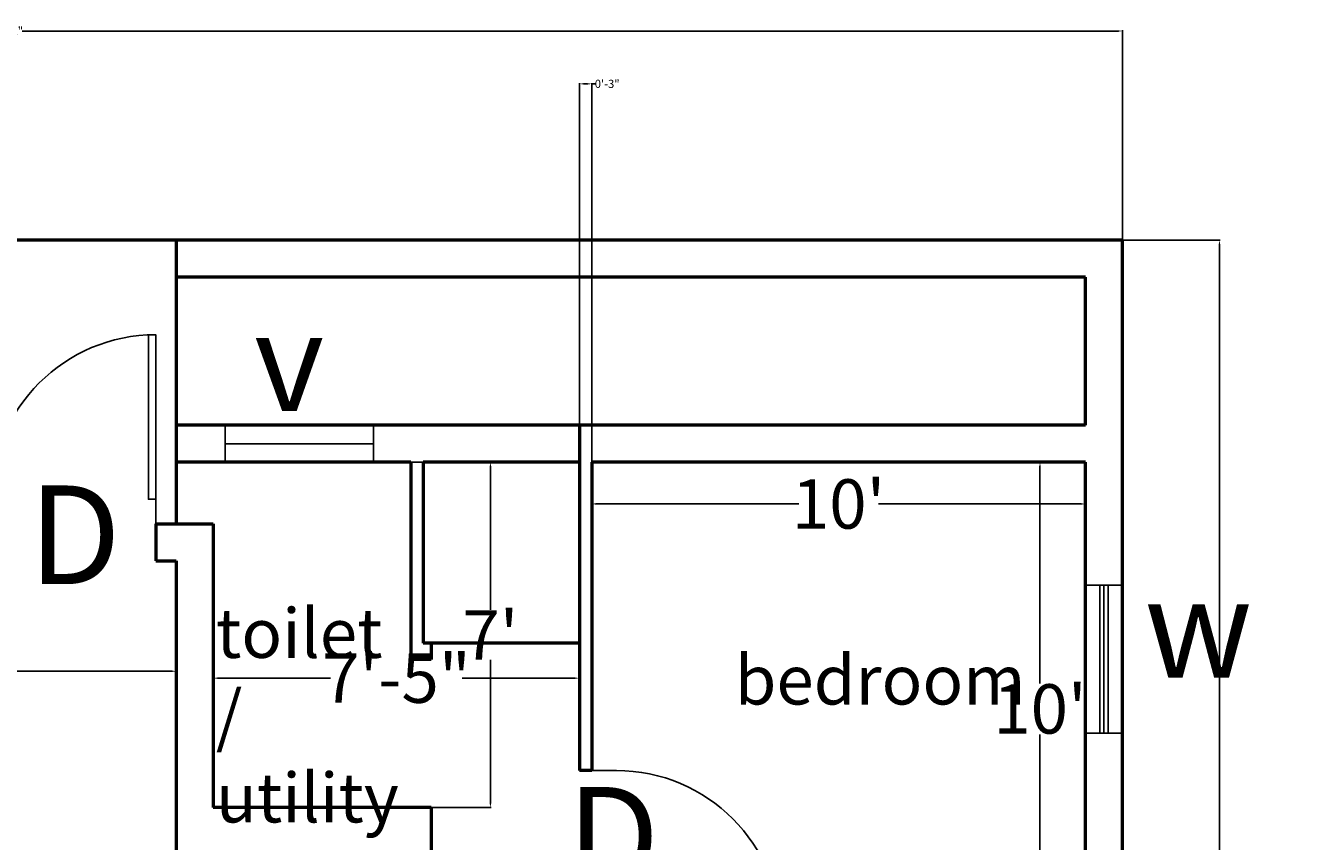
# Model space of a CAD drawing. Units: inches. Extents: x 409 to 7572, y 7 to 725.
# Tile 33 of 38: x 5952 to 6263, y 526 to 725. Entities that reach past the tile are written whole.
import ezdxf

# ---------------------------------------------------------------- set-up
doc = ezdxf.new("R2010")
doc.units = ezdxf.units.IN
doc.header["$MEASUREMENT"] = 0
for name, color, linetype, lineweight in [('A-ANNO-DIMS', 2, 'Continuous', 18), ('A-ANNO-SYMB', 3, 'Continuous', 25), ('A-AREA-IDEN', 7, 'Continuous', 25), ('A-DOOR', 3, 'Continuous', 25), ('A-GLAZ', 4, 'Continuous', 25), ('A-WALL', 7, 'Continuous', 50)]:
    doc.layers.add(name, color=color, linetype=linetype, lineweight=lineweight)
doc.styles.get("Standard").update_dxf_attribs({"font": 'arial.ttf'})
doc.dimstyles.get("Standard").update_dxf_attribs({"dimtxt": 2, "dimasz": 1, "dimexe": 0.18, "dimexo": 0.0625, "dimgap": 0.09, "dimtad": 0, "dimtih": 1, "dimtoh": 1, "dimdec": 0, "dimzin": 0, "dimdsep": 46, "dimlunit": 3, "dimtxsty": 'Standard', "dimcen": 0.09, "dimadec": 0, "dimazin": 0, "dimtfac": 1, "dimtdec": 0, "dimtofl": 0, "dimtmove": 0, "dimatfit": 3, "dimfxl": 1, "dimtolj": 1, "dimtzin": 0, "dimarcsym": 0})

# ---------------------------------------------------------------- blocks, each defined once
blk = doc.blocks.new('*U2')
for p, q in [((0, 0), (0, -6)), ((-40, 0), (-40, -6))]:
    blk.add_line(p, q)
blk.add_lwpolyline([(0, 0), (0, 40), (-1.75, 40), (-1.75, 0)], close=True)
blk.add_arc((0, 0), 40, 90, 180)
blk = doc.blocks.new('*U6')
for p, q in [((0, 0), (0, -6)), ((-40, 0), (-40, -6))]:
    blk.add_line(p, q)
blk.add_lwpolyline([(0, 0), (0, 40), (-1.75, 40), (-1.75, 0)], close=True)
blk.add_arc((0, 0), 40, 90, 180)
blk = doc.blocks.new('*D129')
at = {"layer": 'A-ANNO-DIMS', "color": 0, "lineweight": -2, "transparency": 16777216}
for p, q in [((6089.78, 618.47), (6089.78, 608.19)), ((6209.78, 618.47), (6209.78, 608.19)), ((6090.78, 608.37), (6140.08, 608.37)), ((6208.78, 608.37), (6159.49, 608.37))]:
    blk.add_line(p, q, dxfattribs=at)
at = {"layer": 'A-ANNO-DIMS', "color": 0, "transparency": 16777216}
for points in [[(6090.78, 608.54), (6090.78, 608.2), (6089.78, 608.37)], [(6208.78, 608.54), (6208.78, 608.2), (6209.78, 608.37)]]:
    blk.add_solid(points, dxfattribs=at)
at = {"layer": 'DEFPOINTS', "color": 0, "transparency": 16777216}
for p in [(6089.78, 618.53), (6209.78, 618.53), (6089.78, 608.37)]:
    blk.add_point(p, dxfattribs=at)
at = {"layer": 'A-ANNO-DIMS', "color": 0, "transparency": 16777216, "insert": (6149.78, 608.37), "char_height": 2, "attachment_point": 5}
blk.add_mtext("\\A1;{\\H6x;10'}", dxfattribs=at)
blk = doc.blocks.new('*D130')
at = {"layer": 'A-ANNO-DIMS', "color": 0, "lineweight": -2, "transparency": 16777216}
for p, q in [((6209.72, 618.53), (6198.55, 618.53)), ((6198.73, 617.53), (6198.73, 564.75)), ((6198.73, 499.53), (6198.73, 552.31)), ((6209.72, 498.53), (6198.55, 498.53))]:
    blk.add_line(p, q, dxfattribs=at)
at = {"layer": 'A-ANNO-DIMS', "color": 0, "transparency": 16777216}
for points in [[(6198.57, 617.53), (6198.9, 617.53), (6198.73, 618.53)], [(6198.57, 499.53), (6198.9, 499.53), (6198.73, 498.53)]]:
    blk.add_solid(points, dxfattribs=at)
at = {"layer": 'DEFPOINTS', "color": 0, "transparency": 16777216}
for p in [(6198.73, 618.53), (6209.78, 618.53), (6209.78, 498.53)]:
    blk.add_point(p, dxfattribs=at)
at = {"layer": 'A-ANNO-DIMS', "color": 0, "transparency": 16777216, "insert": (6198.73, 558.53), "char_height": 2, "attachment_point": 5}
blk.add_mtext("\\A1;{\\H6x;10'}", dxfattribs=at)
blk = doc.blocks.new('*D135')
at = {"layer": 'A-ANNO-DIMS', "color": 0, "lineweight": -2, "transparency": 16777216}
for p, q in [((5853.78, 563.4), (5853.78, 567.87)), ((5854.78, 567.69), (5901.15, 567.69)), ((5987.78, 567.69), (5941.42, 567.69)), ((5988.78, 563.4), (5988.78, 567.87))]:
    blk.add_line(p, q, dxfattribs=at)
at = {"layer": 'A-ANNO-DIMS', "color": 0, "transparency": 16777216}
for points in [[(5854.78, 567.86), (5854.78, 567.52), (5853.78, 567.69)], [(5987.78, 567.86), (5987.78, 567.52), (5988.78, 567.69)]]:
    blk.add_solid(points, dxfattribs=at)
at = {"layer": 'DEFPOINTS', "color": 0, "transparency": 16777216}
for p in [(5988.78, 567.69), (5853.78, 563.33), (5988.78, 563.33)]:
    blk.add_point(p, dxfattribs=at)
at = {"layer": 'A-ANNO-DIMS', "color": 0, "transparency": 16777216, "insert": (5921.28, 567.69), "char_height": 2, "attachment_point": 5}
blk.add_mtext('\\A1;{\\H6x;11\'-3"}', dxfattribs=at)
blk = doc.blocks.new('*D141')
at = {"layer": 'A-ANNO-DIMS', "color": 0, "lineweight": -2, "transparency": 16777216}
for p, q in [((5997.78, 568.97), (5997.78, 565.83)), ((6086.78, 568.97), (6086.78, 565.83)), ((5998.78, 566.01), (6026.29, 566.01)), ((6085.78, 566.01), (6058.27, 566.01))]:
    blk.add_line(p, q, dxfattribs=at)
at = {"layer": 'A-ANNO-DIMS', "color": 0, "transparency": 16777216}
for points in [[(5998.78, 566.17), (5998.78, 565.84), (5997.78, 566.01)], [(6085.78, 566.17), (6085.78, 565.84), (6086.78, 566.01)]]:
    blk.add_solid(points, dxfattribs=at)
at = {"layer": 'DEFPOINTS', "color": 0, "transparency": 16777216}
for p in [(5997.78, 569.03), (6086.78, 569.03), (6086.78, 566.01)]:
    blk.add_point(p, dxfattribs=at)
at = {"layer": 'A-ANNO-DIMS', "color": 0, "transparency": 16777216, "insert": (6042.28, 566.01), "char_height": 2, "attachment_point": 5}
blk.add_mtext('\\A1;{\\H6x;7\'-5"}', dxfattribs=at)
blk = doc.blocks.new('*D142')
at = {"layer": 'A-ANNO-DIMS', "color": 0, "lineweight": -2, "transparency": 16777216}
for p, q in [((6017.35, 618.53), (6065.32, 618.53)), ((6065.14, 617.53), (6065.14, 582.62)), ((6065.14, 535.53), (6065.14, 570.44)), ((6017.35, 534.53), (6065.32, 534.53))]:
    blk.add_line(p, q, dxfattribs=at)
at = {"layer": 'A-ANNO-DIMS', "color": 0, "transparency": 16777216}
for points in [[(6064.97, 617.53), (6065.31, 617.53), (6065.14, 618.53)], [(6064.97, 535.53), (6065.31, 535.53), (6065.14, 534.53)]]:
    blk.add_solid(points, dxfattribs=at)
at = {"layer": 'DEFPOINTS', "color": 0, "transparency": 16777216}
for p in [(6017.28, 618.53), (6017.28, 534.53), (6065.14, 534.53)]:
    blk.add_point(p, dxfattribs=at)
at = {"layer": 'A-ANNO-DIMS', "color": 0, "transparency": 16777216, "insert": (6065.14, 576.53), "char_height": 2, "attachment_point": 5}
blk.add_mtext("\\A1;{\\H6x;7'}", dxfattribs=at)
blk = doc.blocks.new('*D146')
at = {"layer": 'A-ANNO-DIMS', "color": 0, "lineweight": -2, "transparency": 16777216}
for p, q in [((5676.78, 672.59), (5676.78, 723.56)), ((5677.78, 723.38), (5944.22, 723.38)), ((6217.78, 723.38), (5951.35, 723.38)), ((6218.78, 672.59), (6218.78, 723.56))]:
    blk.add_line(p, q, dxfattribs=at)
at = {"layer": 'A-ANNO-DIMS', "color": 0, "transparency": 16777216}
for points in [[(5677.78, 723.55), (5677.78, 723.22), (5676.78, 723.38)], [(6217.78, 723.55), (6217.78, 723.22), (6218.78, 723.38)]]:
    blk.add_solid(points, dxfattribs=at)
at = {"layer": 'DEFPOINTS', "color": 0, "transparency": 16777216}
for p in [(5676.78, 723.38), (5676.78, 672.53), (6218.78, 672.53)]:
    blk.add_point(p, dxfattribs=at)
at = {"layer": 'A-ANNO-DIMS', "color": 0, "transparency": 16777216, "insert": (5947.78, 723.38), "char_height": 2, "attachment_point": 5}
blk.add_mtext('\\A1;45\'-2"', dxfattribs=at)
blk = doc.blocks.new('*D148')
at = {"layer": 'A-ANNO-DIMS', "color": 0, "lineweight": -2, "transparency": 16777216}
for p, q in [((6218.85, 672.53), (6242.53, 672.53)), ((6242.35, 671.53), (6242.35, 500.86)), ((6242.35, 316.53), (6242.35, 488.43)), ((6218.85, 315.53), (6242.53, 315.53))]:
    blk.add_line(p, q, dxfattribs=at)
at = {"layer": 'A-ANNO-DIMS', "color": 0, "transparency": 16777216}
for points in [[(6242.18, 671.53), (6242.52, 671.53), (6242.35, 672.53)], [(6242.18, 316.53), (6242.52, 316.53), (6242.35, 315.53)]]:
    blk.add_solid(points, dxfattribs=at)
at = {"layer": 'DEFPOINTS', "color": 0, "transparency": 16777216}
for p in [(6218.78, 672.53), (6242.35, 672.53), (6218.78, 315.53)]:
    blk.add_point(p, dxfattribs=at)
at = {"layer": 'A-ANNO-DIMS', "color": 0, "transparency": 16777216, "insert": (6242.35, 494.65), "char_height": 2, "attachment_point": 5}
blk.add_mtext('\\A1;{\\H6x;29\'-9"}', dxfattribs=at)
blk = doc.blocks.new('WIN-36')
for p, q in [((1699.82, 514.65), (1699.82, 478.65)), ((1700.82, 514.65), (1700.82, 478.65)), ((1701.82, 514.65), (1701.82, 478.65))]:
    blk.add_line(p, q)
blk.add_lwpolyline([(1705.32, 514.65), (1705.32, 478.65), (1696.32, 478.65), (1696.32, 514.65)], close=True)
blk = doc.blocks.new('VENT-36')
blk.add_line((5633.28, 355.73), (5633.28, 391.73))
blk.add_lwpolyline([(5628.78, 355.73), (5628.78, 391.73), (5637.78, 391.73), (5637.78, 355.73)], close=True)
blk = doc.blocks.new('*D194')
at = {"layer": 'A-ANNO-DIMS', "color": 0, "lineweight": -2, "transparency": 16777216}
for p, q in [((6086.78, 627.59), (6086.78, 710.71)), ((6087.78, 710.53), (6088.78, 710.53)), ((6089.78, 618.59), (6089.78, 710.71)), ((6089.78, 710.53), (6090.78, 710.53))]:
    blk.add_line(p, q, dxfattribs=at)
at = {"layer": 'A-ANNO-DIMS', "color": 0, "transparency": 16777216}
for points in [[(6087.78, 710.7), (6087.78, 710.36), (6086.78, 710.53)], [(6088.78, 710.7), (6088.78, 710.36), (6089.78, 710.53)]]:
    blk.add_solid(points, dxfattribs=at)
at = {"layer": 'DEFPOINTS', "color": 0, "transparency": 16777216}
for p in [(6089.78, 710.53), (6086.78, 627.53), (6089.78, 618.53)]:
    blk.add_point(p, dxfattribs=at)
at = {"layer": 'A-ANNO-DIMS', "color": 0, "transparency": 16777216, "insert": (6093.53, 710.53), "char_height": 2, "attachment_point": 5}
blk.add_mtext('\\A1;0\'-3"', dxfattribs=at)

msp = doc.modelspace()

# ---------------------------------------------------------------- linework, layer by layer
at = {"layer": 'A-WALL'}
for p, q in [((6218.78, 672.53), (5676.78, 672.53)), ((5988.78, 672.53), (5988.78, 603.53)), ((6218.78, 315.53), (6218.78, 672.53)), ((6209.78, 663.53), (5988.78, 663.53)), ((6209.78, 627.53), (6209.78, 663.53)), ((6209.78, 627.53), (5988.78, 627.53)), ((6086.78, 627.53), (6086.78, 543.53)), ((6045.78, 618.53), (5988.78, 618.53)), ((6045.78, 618.53), (6045.78, 570.53)), ((6086.78, 618.53), (6048.78, 618.53)), ((6048.78, 618.53), (6048.78, 574.53)), ((6209.78, 618.53), (6089.78, 618.53)), ((6089.78, 618.53), (6089.78, 543.53)), ((6209.78, 498.53), (6209.78, 618.53)), ((5983.78, 603.53), (5997.78, 603.53)), ((5983.78, 603.53), (5983.78, 594.53)), ((5997.78, 603.53), (5997.78, 534.53)), ((5983.78, 594.53), (5988.78, 594.53)), ((6086.78, 574.53), (6048.78, 574.53)), ((6050.78, 574.53), (6050.78, 570.53)), ((6050.78, 570.53), (6045.78, 570.53)), ((6089.78, 543.53), (6086.78, 543.53)), ((6050.78, 534.53), (5997.78, 534.53)), ((6050.78, 534.53), (6050.78, 453.53))]:
    msp.add_line(p, q, dxfattribs=at)
msp.add_lwpolyline([(5988.78, 594.53), (5988.78, 525.53), (5988.78, 469.53)], dxfattribs=at)

# ---------------------------------------------------------------- block references
at = {"layer": 'A-DOOR'}
msp.add_blockref('*U2', (5983.78, 609.53), dxfattribs=at)
at = {"layer": 'A-DOOR', "rotation": 270}
msp.add_blockref('*U6', (6095.78, 503.53), dxfattribs=at)
at = {"layer": 'A-GLAZ', "rotation": 269.9999999999993}
msp.add_blockref('VENT-36', (5644.97, 6256.31), dxfattribs=at)
at = {"layer": 'A-GLAZ'}
msp.add_blockref('WIN-36', (4513.46, 73.99), dxfattribs=at)

# ---------------------------------------------------------------- texts
at = {"layer": 'A-ANNO-SYMB', "char_height": 24, "attachment_point": 1}
for s, width, insert in [('v', 18.2582, (6007.69, 654.94)), ('D', 19.1972, (5952.81, 612.87)), ('w', 18.2582, (6224.09, 590.15)), ('D', 19.1972, (6083.71, 539.54))]:
    msp.add_mtext_dynamic_manual_height_columns(s, width=width, gutter_width=1, heights=[0], dxfattribs=dict(at, insert=insert))
at = {"layer": 'A-AREA-IDEN', "char_height": 12, "attachment_point": 1}
for s, width, insert in [('toilet / utility', 49.2946, (5998.43, 582.94)), ('bedroom', 40.9017, (6124.54, 571.6))]:
    msp.add_mtext_dynamic_manual_height_columns(s, width=width, gutter_width=1, heights=[0], dxfattribs=dict(at, insert=insert))

# ---------------------------------------------------------------- dimensions: what is measured, and where the dimension line sits
at = {"layer": 'A-ANNO-DIMS'}
for base, p1, p2, override, picture, middle in [((5676.78, 723.38), (6218.78, 672.53), (5676.78, 672.53), {"dimclrd": 0, "dimclre": 0, "dimclrt": 0}, '*D146', (5947.78, 723.38)), ((6089.78, 710.53), (6086.78, 627.53), (6089.78, 618.53), {"dimdec": 1, "dimlfac": 1, "dimrnd": 0, "dimzin": 1, "dimdsep": 46, "dimlunit": 4, "dimfrac": 2}, '*D194', (6093.53, 710.53))]:
    dim = msp.add_linear_dim(base=base, p1=p1, p2=p2, dimstyle='Standard', override=override, dxfattribs=at)
    dim.commit()
    dim.dimension.update_dxf_attribs({"geometry": picture, "text_midpoint": middle})
dim = msp.add_linear_dim(base=(6242.35, 672.53), p1=(6218.78, 315.53), p2=(6218.78, 672.53), angle=90, text='{\\H6x;<>}', dimstyle='Standard', override={"dimclrd": 0, "dimclre": 0, "dimclrt": 0}, dxfattribs=at)
dim.commit()
dim.dimension.update_dxf_attribs({"geometry": '*D148', "text_midpoint": (6242.35, 494.65), "dimtype": 160})
for base, p1, p2, picture, middle in [((6065.14, 534.53), (6017.28, 618.53), (6017.28, 534.53), '*D142', (6065.14, 576.53)), ((6198.73, 618.53), (6209.78, 498.53), (6209.78, 618.53), '*D130', (6198.73, 558.53))]:
    dim = msp.add_linear_dim(base=base, p1=p1, p2=p2, angle=90, text='{\\H6x;<>}', dimstyle='Standard', override={"dimclrd": 0, "dimclre": 0, "dimclrt": 0}, dxfattribs=at)
    dim.commit()
    dim.dimension.update_dxf_attribs({"geometry": picture, "text_midpoint": middle})
for base, p1, p2, picture, middle in [((6089.78, 608.37), (6209.78, 618.53), (6089.78, 618.53), '*D129', (6149.78, 608.37)), ((5988.78, 567.69), (5853.78, 563.33), (5988.78, 563.33), '*D135', (5921.28, 567.69)), ((6086.78, 566.01), (5997.78, 569.03), (6086.78, 569.03), '*D141', (6042.28, 566.01))]:
    dim = msp.add_linear_dim(base=base, p1=p1, p2=p2, text='{\\H6x;<>}', dimstyle='Standard', override={"dimclrd": 0, "dimclre": 0, "dimclrt": 0}, dxfattribs=at)
    dim.commit()
    dim.dimension.update_dxf_attribs({"geometry": picture, "text_midpoint": middle})

doc.saveas('drawing.dxf')
